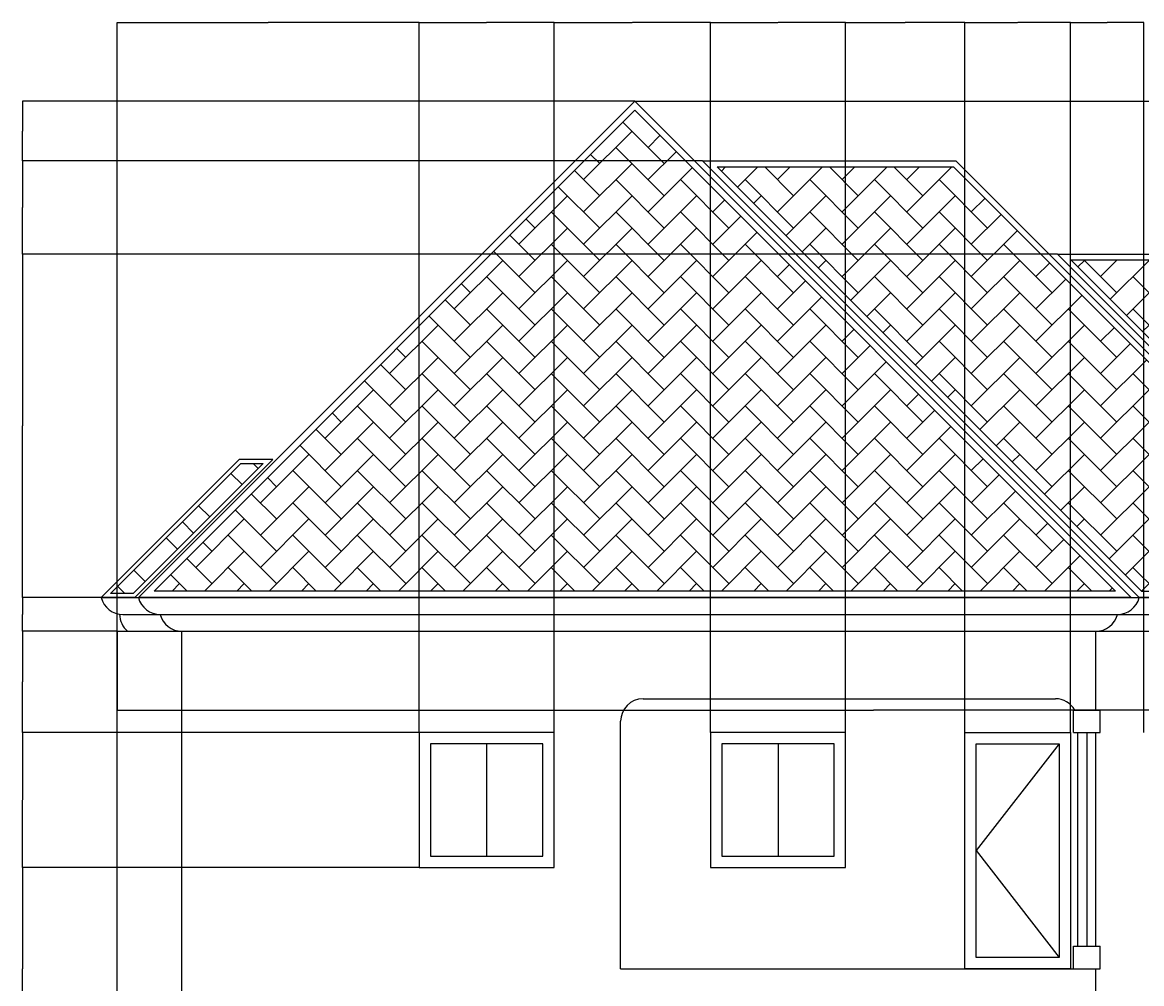
# Model space of a CAD drawing. Units: millimetres. Extents: x 19292 to 100733, y 12374 to 26974.
# Tile 24 of 24: x 85594 to 95547, y 18427 to 26974. Entities that reach past the tile are written whole.
import ezdxf

# ---------------------------------------------------------------- set-up
doc = ezdxf.new("R2010")
doc.units = ezdxf.units.MM
for name, color, linetype, lineweight in [('A-ANNO-DIMS', 2, 'Continuous', 18), ('A-ELEV', 7, 'Continuous', 25), ('A-ELEV-PATT', 8, 'Continuous', 13)]:
    doc.layers.add(name, color=color, linetype=linetype, lineweight=lineweight)
doc.styles.get("Standard").update_dxf_attribs({"font": 'arial.ttf'})
doc.dimstyles.get("Standard").update_dxf_attribs({"dimtxt": 0.18, "dimasz": 0.18, "dimexe": 0.18, "dimexo": 0.0625, "dimgap": 0.09, "dimtad": 0, "dimtih": 1, "dimtoh": 1, "dimdec": 4, "dimzin": 0, "dimdsep": 46, "dimtxsty": 'Standard', "dimcen": 0.09, "dimadec": 0, "dimazin": 0, "dimtfac": 1, "dimtdec": 4, "dimtofl": 0, "dimtmove": 0, "dimatfit": 3, "dimfxl": 1, "dimtolj": 1, "dimtzin": 0, "dimarcsym": 0})

# ---------------------------------------------------------------- blocks, each defined once
blk = doc.blocks.new('WIN-ELEV-1200')
blk.add_line((599.9999832836038, 1100.000156100592), (599.9999832836038, 100.000156100592))
for points in [[(1199.999983283604, 1200.000156100592), (1199.999983283604, 0.0001561005919939), (-1.67163962033e-05, 0.0001561005919939), (-1.67163962033e-05, 1200.000156100592)], [(1099.999983283604, 1100.000156100592), (1099.999983283604, 100.000156100592), (99.9999832836038, 100.000156100592), (99.9999832836038, 1100.000156100592)]]:
    blk.add_lwpolyline(points, close=True)
blk = doc.blocks.new('*D144')
at = {"layer": 'A-ANNO-DIMS', "color": 0, "lineweight": -2, "transparency": 16777216}
for p, q in [((89121.76770300003, 19459.90915600001), (85593.98509100005, 19459.90915600001)), ((85594.16509100008, 19459.72915600001), (85594.16509100008, 18560.0910591378)), ((85594.16509100008, 17660.08915600001), (85594.16509100008, 18559.72725286222)), ((89236.95448300001, 17659.90915600001), (85593.98509100005, 17659.90915600001))]:
    blk.add_line(p, q, dxfattribs=at)
at = {"layer": 'A-ANNO-DIMS', "color": 0, "transparency": 16777216}
for points in [[(85594.13509100005, 19459.72915600001), (85594.19509100006, 19459.72915600001), (85594.16509100008, 19459.90915600001)], [(85594.13509100005, 17660.08915600001), (85594.19509100006, 17660.08915600001), (85594.16509100008, 17659.90915600001)]]:
    blk.add_solid(points, dxfattribs=at)
at = {"layer": 'Defpoints', "color": 0, "transparency": 16777216}
for p in [(85594.16509100008, 19459.90915600001), (89121.83020300003, 19459.90915600001), (89237.01698300002, 17659.90915600001)]:
    blk.add_point(p, dxfattribs=at)
at = {"layer": 'A-ANNO-DIMS', "color": 0, "transparency": 16777216, "insert": (85594.16509100005, 18559.90915599998), "char_height": 0.18, "attachment_point": 5}
blk.add_mtext('\\A1;1800', dxfattribs=at)
blk = doc.blocks.new('*D145')
at = {"layer": 'A-ANNO-DIMS', "color": 0, "lineweight": -2, "transparency": 16777216}
for p, q in [((89121.76770300003, 20659.90915600001), (85593.98509100005, 20659.90915600001)), ((85594.16509100008, 20659.72915600001), (85594.16509100008, 20060.0910591378)), ((85594.16509100008, 19460.08915600001), (85594.16509100008, 20059.72725286222)), ((89121.76770300003, 19459.90915600001), (85593.98509100005, 19459.90915600001))]:
    blk.add_line(p, q, dxfattribs=at)
at = {"layer": 'A-ANNO-DIMS', "color": 0, "transparency": 16777216}
for points in [[(85594.13509100005, 20659.72915600001), (85594.19509100006, 20659.72915600001), (85594.16509100008, 20659.90915600001)], [(85594.13509100005, 19460.08915600001), (85594.19509100006, 19460.08915600001), (85594.16509100008, 19459.90915600001)]]:
    blk.add_solid(points, dxfattribs=at)
at = {"layer": 'Defpoints', "color": 0, "transparency": 16777216}
for p in [(85594.16509100008, 20659.90915600001), (89121.83020300003, 20659.90915600001), (89121.83020300003, 19459.90915600001)]:
    blk.add_point(p, dxfattribs=at)
at = {"layer": 'A-ANNO-DIMS', "color": 0, "transparency": 16777216, "insert": (85594.16509100005, 20059.90915599999), "char_height": 0.18, "attachment_point": 5}
blk.add_mtext('\\A1;1200', dxfattribs=at)
blk = doc.blocks.new('*D146')
at = {"layer": 'A-ANNO-DIMS', "color": 0, "lineweight": -2, "transparency": 16777216}
for p, q in [((86437.75175800003, 21559.90915600001), (85593.98509100005, 21559.90915600001)), ((85594.16509100008, 21559.72915600001), (85594.16509100008, 21110.0910591378)), ((85594.16509100008, 20660.08915600001), (85594.16509100008, 21109.72725286222)), ((89121.76770300003, 20659.90915600001), (85593.98509100005, 20659.90915600001))]:
    blk.add_line(p, q, dxfattribs=at)
at = {"layer": 'A-ANNO-DIMS', "color": 0, "transparency": 16777216}
for points in [[(85594.13509100005, 21559.72915600001), (85594.19509100006, 21559.72915600001), (85594.16509100008, 21559.90915600001)], [(85594.13509100005, 20660.08915600001), (85594.19509100006, 20660.08915600001), (85594.16509100008, 20659.90915600001)]]:
    blk.add_solid(points, dxfattribs=at)
at = {"layer": 'Defpoints', "color": 0, "transparency": 16777216}
for p in [(85594.16509100008, 21559.90915600001), (86437.81425800003, 21559.90915600001), (89121.83020300003, 20659.90915600001)]:
    blk.add_point(p, dxfattribs=at)
at = {"layer": 'A-ANNO-DIMS', "color": 0, "transparency": 16777216, "insert": (85594.16509100005, 21109.90915599999), "char_height": 0.18, "attachment_point": 5}
blk.add_mtext('\\A1;900', dxfattribs=at)
blk = doc.blocks.new('*D147')
at = {"layer": 'A-ANNO-DIMS', "color": 0, "lineweight": -2, "transparency": 16777216}
for p, q in [((86294.10259100003, 21859.90915600001), (85593.98509100005, 21859.90915600001)), ((85594.16509100008, 21859.72915600001), (85594.16509100008, 21710.09112052934)), ((85594.16509100008, 21560.08915600001), (85594.16509100008, 21709.72719147068)), ((86437.75175800003, 21559.90915600001), (85593.98509100005, 21559.90915600001))]:
    blk.add_line(p, q, dxfattribs=at)
at = {"layer": 'A-ANNO-DIMS', "color": 0, "transparency": 16777216}
for points in [[(85594.13509100005, 21859.72915600001), (85594.19509100006, 21859.72915600001), (85594.16509100008, 21859.90915600001)], [(85594.13509100005, 21560.08915600001), (85594.19509100006, 21560.08915600001), (85594.16509100008, 21559.90915600001)]]:
    blk.add_solid(points, dxfattribs=at)
at = {"layer": 'Defpoints', "color": 0, "transparency": 16777216}
for p in [(85594.16509100008, 21859.90915600001), (86294.16509100003, 21859.90915600001), (86437.81425800003, 21559.90915600001)]:
    blk.add_point(p, dxfattribs=at)
at = {"layer": 'A-ANNO-DIMS', "color": 0, "transparency": 16777216, "insert": (85594.16509100005, 21709.90915599998), "char_height": 0.18, "attachment_point": 5}
blk.add_mtext('\\A1;300', dxfattribs=at)
blk = doc.blocks.new('*D148')
at = {"layer": 'A-ANNO-DIMS', "color": 0, "lineweight": -2, "transparency": 16777216}
for p, q in [((94798.25936700004, 24912.22737000001), (85593.98509100005, 24912.22737000001)), ((85594.16509100008, 24912.04737000001), (85594.16509100008, 23386.25022752934)), ((85594.16509100008, 21860.08915600001), (85594.16509100008, 23385.88629847067)), ((86294.10259100003, 21859.90915600001), (85593.98509100005, 21859.90915600001))]:
    blk.add_line(p, q, dxfattribs=at)
at = {"layer": 'A-ANNO-DIMS', "color": 0, "transparency": 16777216}
for points in [[(85594.13509100005, 24912.04737000001), (85594.19509100006, 24912.04737000001), (85594.16509100008, 24912.22737000001)], [(85594.13509100005, 21860.08915600001), (85594.19509100006, 21860.08915600001), (85594.16509100008, 21859.90915600001)]]:
    blk.add_solid(points, dxfattribs=at)
at = {"layer": 'Defpoints', "color": 0, "transparency": 16777216}
for p in [(85594.16509100008, 24912.22737000001), (94798.32186700004, 24912.22737000001), (86294.16509100003, 21859.90915600001)]:
    blk.add_point(p, dxfattribs=at)
at = {"layer": 'A-ANNO-DIMS', "color": 0, "transparency": 16777216, "insert": (85594.16509100005, 23386.06826299999), "char_height": 0.18, "attachment_point": 5}
blk.add_mtext('\\A1;3052.3', dxfattribs=at)
blk = doc.blocks.new('*D149')
at = {"layer": 'A-ANNO-DIMS', "color": 0, "lineweight": -2, "transparency": 16777216}
for p, q in [((91642.59139800003, 25742.60711800001), (85593.98509100005, 25742.60711800001)), ((85594.16509100008, 25742.42711800001), (85594.16509100008, 25327.59920852934)), ((85594.16509100008, 24912.40737000001), (85594.16509100008, 25327.23527947068)), ((94798.25936700004, 24912.22737000001), (85593.98509100005, 24912.22737000001))]:
    blk.add_line(p, q, dxfattribs=at)
at = {"layer": 'A-ANNO-DIMS', "color": 0, "transparency": 16777216}
for points in [[(85594.13509100005, 25742.42711800001), (85594.19509100006, 25742.42711800001), (85594.16509100008, 25742.60711800001)], [(85594.13509100005, 24912.40737000001), (85594.19509100006, 24912.40737000001), (85594.16509100008, 24912.22737000001)]]:
    blk.add_solid(points, dxfattribs=at)
at = {"layer": 'Defpoints', "color": 0, "transparency": 16777216}
for p in [(85594.16509100008, 25742.60711800001), (91642.65389800003, 25742.60711800001), (94798.32186700004, 24912.22737000001)]:
    blk.add_point(p, dxfattribs=at)
at = {"layer": 'A-ANNO-DIMS', "color": 0, "transparency": 16777216, "insert": (85594.16509100005, 25327.41724399998), "char_height": 0.18, "attachment_point": 5}
blk.add_mtext('\\A1;830.4', dxfattribs=at)
blk = doc.blocks.new('*D150')
at = {"layer": 'A-ANNO-DIMS', "color": 0, "lineweight": -2, "transparency": 16777216}
for p, q in [((91039.43747500001, 26274.21100900001), (85593.98509100005, 26274.21100900001)), ((85594.16509100008, 26274.03100900001), (85594.16509100008, 26008.59102802934)), ((85594.16509100008, 25742.78711800001), (85594.16509100008, 26008.22709897068)), ((91642.59139800003, 25742.60711800001), (85593.98509100005, 25742.60711800001))]:
    blk.add_line(p, q, dxfattribs=at)
at = {"layer": 'A-ANNO-DIMS', "color": 0, "transparency": 16777216}
for points in [[(85594.13509100005, 26274.03100900001), (85594.19509100006, 26274.03100900001), (85594.16509100008, 26274.21100900001)], [(85594.13509100005, 25742.78711800001), (85594.19509100006, 25742.78711800001), (85594.16509100008, 25742.60711800001)]]:
    blk.add_solid(points, dxfattribs=at)
at = {"layer": 'Defpoints', "color": 0, "transparency": 16777216}
for p in [(85594.16509100008, 26274.21100900001), (91039.49997500001, 26274.21100900001), (91642.65389800003, 25742.60711800001)]:
    blk.add_point(p, dxfattribs=at)
at = {"layer": 'A-ANNO-DIMS', "color": 0, "transparency": 16777216, "insert": (85594.16509100005, 26008.40906349998), "char_height": 0.18, "attachment_point": 5}
blk.add_mtext('\\A1;531.6', dxfattribs=at)
blk = doc.blocks.new('*D151')
at = {"layer": 'A-ANNO-DIMS', "color": 0, "lineweight": -2, "transparency": 16777216}
for p, q in [((91039.56247500001, 26274.21100900001), (100732.6942110001, 26274.21100900001)), ((100732.5142110001, 26274.03100900001), (100732.5142110001, 20692.2419856378)), ((100732.5142110001, 15110.08915600001), (100732.5142110001, 20691.87817936222)), ((99927.91327500006, 15109.909156), (100732.6942110001, 15109.909156))]:
    blk.add_line(p, q, dxfattribs=at)
at = {"layer": 'A-ANNO-DIMS', "color": 0, "transparency": 16777216}
for points in [[(100732.4842110001, 26274.03100900001), (100732.5442110001, 26274.03100900001), (100732.5142110001, 26274.21100900001)], [(100732.4842110001, 15110.08915600001), (100732.5442110001, 15110.08915600001), (100732.5142110001, 15109.909156)]]:
    blk.add_solid(points, dxfattribs=at)
at = {"layer": 'Defpoints', "color": 0, "transparency": 16777216}
for p in [(91039.49997500001, 26274.21100900001), (100732.5142110001, 26274.21100900001), (99927.85077500006, 15109.909156)]:
    blk.add_point(p, dxfattribs=at)
at = {"layer": 'A-ANNO-DIMS', "color": 0, "transparency": 16777216, "insert": (100732.5142110001, 20692.06008249997), "char_height": 0.18, "attachment_point": 5}
blk.add_mtext('\\A1;11164', dxfattribs=at)
blk = doc.blocks.new('*D161')
at = {"layer": 'A-ANNO-DIMS', "color": 0, "lineweight": -2, "transparency": 16777216}
for p, q in [((86437.814258, 21559.971656), (86437.814258, 26974.391009)), ((86437.99425799999, 26974.211009), (87779.46229189154, 26974.211009)), ((89121.65020300001, 26974.211009), (87780.18216910846, 26974.211009)), ((89121.830203, 20659.971656), (89121.830203, 26974.391009))]:
    blk.add_line(p, q, dxfattribs=at)
at = {"layer": 'A-ANNO-DIMS', "color": 0, "transparency": 16777216}
for points in [[(86437.99425799999, 26974.241009), (86437.99425799999, 26974.181009), (86437.814258, 26974.211009)], [(89121.65020300001, 26974.241009), (89121.65020300001, 26974.181009), (89121.830203, 26974.211009)]]:
    blk.add_solid(points, dxfattribs=at)
at = {"layer": 'Defpoints', "color": 0, "transparency": 16777216}
for p in [(89121.830203, 26974.211009), (86437.814258, 21559.909156), (89121.830203, 20659.909156)]:
    blk.add_point(p, dxfattribs=at)
at = {"layer": 'A-ANNO-DIMS', "color": 0, "transparency": 16777216, "insert": (87779.8222305, 26974.211009), "char_height": 0.18, "attachment_point": 5}
blk.add_mtext('\\A1;2684', dxfattribs=at)
blk = doc.blocks.new('*D162')
at = {"layer": 'A-ANNO-DIMS', "color": 0, "lineweight": -2, "transparency": 16777216}
for p, q in [((89121.830203, 20659.971656), (89121.830203, 26974.391009)), ((89122.01020299998, 26974.211009), (89721.48020982128, 26974.211009)), ((90321.650203, 26974.211009), (89722.18019617873, 26974.211009)), ((90321.830203, 20659.971656), (90321.830203, 26974.391009))]:
    blk.add_line(p, q, dxfattribs=at)
at = {"layer": 'A-ANNO-DIMS', "color": 0, "transparency": 16777216}
for points in [[(89122.01020299998, 26974.241009), (89122.01020299998, 26974.181009), (89121.830203, 26974.211009)], [(90321.650203, 26974.241009), (90321.650203, 26974.181009), (90321.830203, 26974.211009)]]:
    blk.add_solid(points, dxfattribs=at)
at = {"layer": 'Defpoints', "color": 0, "transparency": 16777216}
for p in [(90321.830203, 26974.211009), (89121.830203, 20659.909156), (90321.830203, 20659.909156)]:
    blk.add_point(p, dxfattribs=at)
at = {"layer": 'A-ANNO-DIMS', "color": 0, "transparency": 16777216, "insert": (89721.830203, 26974.211009), "char_height": 0.18, "attachment_point": 5}
blk.add_mtext('\\A1;1200', dxfattribs=at)
blk = doc.blocks.new('*D163')
at = {"layer": 'A-ANNO-DIMS', "color": 0, "lineweight": -2, "transparency": 16777216}
for p, q in [((90321.830203, 20659.971656), (90321.830203, 26974.391009)), ((90322.010203, 26974.211009), (91017.16552300206, 26974.211009)), ((91713.23103400003, 26974.211009), (91018.07571399795, 26974.211009)), ((91713.411034, 20659.971656), (91713.411034, 26974.391009))]:
    blk.add_line(p, q, dxfattribs=at)
at = {"layer": 'A-ANNO-DIMS', "color": 0, "transparency": 16777216}
for points in [[(90322.010203, 26974.241009), (90322.010203, 26974.181009), (90321.830203, 26974.211009)], [(91713.23103400003, 26974.241009), (91713.23103400003, 26974.181009), (91713.411034, 26974.211009)]]:
    blk.add_solid(points, dxfattribs=at)
at = {"layer": 'Defpoints', "color": 0, "transparency": 16777216}
for p in [(91713.411034, 26974.211009), (90321.830203, 20659.909156), (91713.411034, 20659.909156)]:
    blk.add_point(p, dxfattribs=at)
at = {"layer": 'A-ANNO-DIMS', "color": 0, "transparency": 16777216, "insert": (91017.6206185, 26974.211009), "char_height": 0.18, "attachment_point": 5}
blk.add_mtext('\\A1;1391.6', dxfattribs=at)
blk = doc.blocks.new('*D164')
at = {"layer": 'A-ANNO-DIMS', "color": 0, "lineweight": -2, "transparency": 16777216}
for p, q in [((91713.411034, 20659.971656), (91713.411034, 26974.391009)), ((91713.591034, 26974.211009), (92313.06104082127, 26974.211009)), ((92913.23103400001, 26974.211009), (92313.76102717873, 26974.211009)), ((92913.411034, 20659.971656), (92913.411034, 26974.391009))]:
    blk.add_line(p, q, dxfattribs=at)
at = {"layer": 'A-ANNO-DIMS', "color": 0, "transparency": 16777216}
for points in [[(91713.591034, 26974.241009), (91713.591034, 26974.181009), (91713.411034, 26974.211009)], [(92913.23103400001, 26974.241009), (92913.23103400001, 26974.181009), (92913.411034, 26974.211009)]]:
    blk.add_solid(points, dxfattribs=at)
at = {"layer": 'Defpoints', "color": 0, "transparency": 16777216}
for p in [(92913.411034, 26974.211009), (91713.411034, 20659.909156), (92913.411034, 20659.909156)]:
    blk.add_point(p, dxfattribs=at)
at = {"layer": 'A-ANNO-DIMS', "color": 0, "transparency": 16777216, "insert": (92313.411034, 26974.211009), "char_height": 0.18, "attachment_point": 5}
blk.add_mtext('\\A1;1200', dxfattribs=at)
blk = doc.blocks.new('*D165')
at = {"layer": 'A-ANNO-DIMS', "color": 0, "lineweight": -2, "transparency": 16777216}
for p, q in [((92913.411034, 20659.971656), (92913.411034, 26974.391009)), ((92913.59103399998, 26974.211009), (93443.86200193588, 26974.211009)), ((93975.04365200001, 26974.211009), (93444.77268406413, 26974.211009)), ((93975.223652, 20659.971656), (93975.223652, 26974.391009))]:
    blk.add_line(p, q, dxfattribs=at)
at = {"layer": 'A-ANNO-DIMS', "color": 0, "transparency": 16777216}
for points in [[(92913.59103399998, 26974.241009), (92913.59103399998, 26974.181009), (92913.411034, 26974.211009)], [(93975.04365200001, 26974.241009), (93975.04365200001, 26974.181009), (93975.223652, 26974.211009)]]:
    blk.add_solid(points, dxfattribs=at)
at = {"layer": 'Defpoints', "color": 0, "transparency": 16777216}
for p in [(93975.223652, 26974.211009), (92913.411034, 20659.909156), (93975.223652, 20659.909156)]:
    blk.add_point(p, dxfattribs=at)
at = {"layer": 'A-ANNO-DIMS', "color": 0, "transparency": 16777216, "insert": (93444.317343, 26974.211009), "char_height": 0.18, "attachment_point": 5}
blk.add_mtext('\\A1;1061.8', dxfattribs=at)
blk = doc.blocks.new('*D166')
at = {"layer": 'A-ANNO-DIMS', "color": 0, "lineweight": -2, "transparency": 16777216}
for p, q in [((93975.223652, 20659.971656), (93975.223652, 26974.391009)), ((93975.403652, 26974.211009), (94443.90636884993, 26974.211009)), ((94913.16174600001, 26974.211009), (94444.65902915008, 26974.211009)), ((94913.341746, 20659.971656), (94913.341746, 26974.391009))]:
    blk.add_line(p, q, dxfattribs=at)
at = {"layer": 'A-ANNO-DIMS', "color": 0, "transparency": 16777216}
for points in [[(93975.403652, 26974.241009), (93975.403652, 26974.181009), (93975.223652, 26974.211009)], [(94913.16174600001, 26974.241009), (94913.16174600001, 26974.181009), (94913.341746, 26974.211009)]]:
    blk.add_solid(points, dxfattribs=at)
at = {"layer": 'Defpoints', "color": 0, "transparency": 16777216}
for p in [(94913.341746, 26974.211009), (93975.223652, 20659.909156), (94913.341746, 20659.909156)]:
    blk.add_point(p, dxfattribs=at)
at = {"layer": 'A-ANNO-DIMS', "color": 0, "transparency": 16777216, "insert": (94444.282699, 26974.211009), "char_height": 0.18, "attachment_point": 5}
blk.add_mtext('\\A1;938.1', dxfattribs=at)
blk = doc.blocks.new('*D167')
at = {"layer": 'A-ANNO-DIMS', "color": 0, "lineweight": -2, "transparency": 16777216}
for p, q in [((94913.341746, 20659.971656), (94913.341746, 26974.391009)), ((94913.52174600001, 26974.211009), (95240.02142701363, 26974.211009)), ((95567.099048, 26974.211009), (95240.59936698635, 26974.211009)), ((95567.279048, 20659.971656), (95567.279048, 26974.391009))]:
    blk.add_line(p, q, dxfattribs=at)
at = {"layer": 'A-ANNO-DIMS', "color": 0, "transparency": 16777216}
for points in [[(94913.52174600001, 26974.241009), (94913.52174600001, 26974.181009), (94913.341746, 26974.211009)], [(95567.099048, 26974.241009), (95567.099048, 26974.181009), (95567.279048, 26974.211009)]]:
    blk.add_solid(points, dxfattribs=at)
at = {"layer": 'Defpoints', "color": 0, "transparency": 16777216}
for p in [(95567.279048, 26974.211009), (94913.341746, 20659.909156), (95567.279048, 20659.909156)]:
    blk.add_point(p, dxfattribs=at)
at = {"layer": 'A-ANNO-DIMS', "color": 0, "transparency": 16777216, "insert": (95240.310397, 26974.211009), "char_height": 0.18, "attachment_point": 5}
blk.add_mtext('\\A1;654', dxfattribs=at)
blk = doc.blocks.new('*D170')
at = {"layer": 'A-ANNO-DIMS', "color": 0, "lineweight": -2, "transparency": 16777216}
for p, q in [((86437.814258, 21559.846656), (86437.814258, 20859.729156)), ((99888.865044, 21559.846656), (99888.865044, 20859.729156)), ((86437.99425799999, 20859.909156), (93162.93679970397, 20859.909156)), ((99888.685044, 20859.909156), (93163.74250229605, 20859.909156))]:
    blk.add_line(p, q, dxfattribs=at)
at = {"layer": 'A-ANNO-DIMS', "color": 0, "transparency": 16777216}
for points in [[(86437.99425799999, 20859.939156), (86437.99425799999, 20859.879156), (86437.814258, 20859.909156)], [(99888.685044, 20859.939156), (99888.685044, 20859.879156), (99888.865044, 20859.909156)]]:
    blk.add_solid(points, dxfattribs=at)
at = {"layer": 'Defpoints', "color": 0, "transparency": 16777216}
for p in [(86437.814258, 21559.909156), (99888.865044, 21559.909156), (86437.814258, 20859.909156)]:
    blk.add_point(p, dxfattribs=at)
at = {"layer": 'A-ANNO-DIMS', "color": 0, "transparency": 16777216, "insert": (93163.339651, 20859.909156), "char_height": 0.18, "attachment_point": 5}
blk.add_mtext('\\A1;13451', dxfattribs=at)

msp = doc.modelspace()

# ---------------------------------------------------------------- hatches: boundary and pattern name
at = {"layer": 'A-ELEV-PATT'}
h = msp.add_hatch(dxfattribs=at)
h.set_pattern_fill('AR-HBONE', color=256, scale=2)
h.set_pattern_definition([(45, (-15742.66734838602, 1.819e-12), (0, 287.3681958742129), [609.6, -203.2]), (135, (-15598.98334838602, 143.6840000000018), (2.84e-14, 287.3681958742129), [609.6, -203.2])])
h.paths.add_polyline_path([(87735.48117691663, 23052.98438420805), (87536.44885016952, 23052.98438420805), (86378.42981350586, 21894.96534754441), (86578.07896417224, 21895.58217146364)])
h.paths.add_polyline_path([(91039.49997476467, 26192.70967510026), (86764.32960140108, 21917.5393017367), (95314.67034812817, 21917.5393017367)])
h.paths.add_polyline_path([(93872.96419886049, 25688.93910166301), (91772.21995210611, 25688.939101663), (95547.96497158404, 21913.19408218505), (97648.70921833848, 21913.19408218505)])
h.paths.add_polyline_path([(96958.92150424178, 24862.64804519888), (94918.01694600363, 24862.64804519888), (97871.17317701879, 21909.49181418373), (99911.74658381855, 21909.82296562213)])

# ---------------------------------------------------------------- linework, layer by layer
at = {"layer": 'A-ELEV'}
for p, q in [((91642.65389804375, 25742.60711847878), (93895.19421929128, 25742.60711847879)), ((87819.48539444181, 23087.78007040352), (87522.03600503529, 23087.78007040352)), ((86294.16509073348, 21859.90915610059), (100032.5142111294, 21859.90915610059)), ((86487.81425804386, 21709.9091561006), (99838.86504381908, 21709.90915610059)), ((86437.81425804387, 18559.90915610059), (86437.81425804387, 21559.90915610059)), ((86437.81425804387, 21559.90915610059), (99888.8650438191, 21559.90915610059)), ((87012.49645682552, 15559.90915610059), (87012.49645682552, 21559.90915610059)), ((95138.48032185201, 20859.90915610059), (95138.48032185201, 21559.90915610059)), ((91113.34174630335, 20959.90915610059), (94780.028686983, 20959.90915610059)), ((94940.02868698297, 20859.90915610059), (95178.48032185201, 20859.90915610059)), ((94940.02868698297, 20659.90915610059), (94940.02868698297, 20859.90915610059)), ((95178.48032185201, 20659.90915610059), (95178.48032185201, 20859.90915610059)), ((90913.34174630335, 18559.90915610059), (90913.34174630335, 20759.90915610059)), ((94940.02868698297, 20659.90915610059), (95178.48032185201, 20659.90915610059)), ((94980.02868698302, 18759.90915610059), (94980.02868698302, 20659.90915610059)), ((95059.25450441749, 20659.90915610059), (95059.2545044175, 18759.90915610059)), ((95138.48032185201, 18759.90915610059), (95138.48032185201, 20659.90915610059)), ((94813.34174630335, 20559.90915610059), (94075.22365204261, 19609.90915610059)), ((94075.22365204261, 19609.90915610059), (94813.34174630335, 18659.90915610059)), ((94940.02868698302, 18559.90915610059), (94940.02868698302, 18759.90915610059)), ((94940.02868698302, 18759.90915610059), (95178.48032185201, 18759.90915610059)), ((95178.48032185201, 18559.90915610059), (95178.48032185201, 18759.90915610059)), ((86437.81425804387, 15559.90915610059), (86437.81425804387, 18559.90915610059)), ((90913.34174630335, 18559.90915610059), (94940.02868698302, 18559.90915610059)), ((93975.22365204261, 18559.90915610059), (95178.48032185201, 18559.90915610059)), ((93975.22365204261, 18559.90915610059), (95178.48032185201, 18559.90915610059)), ((95138.48032185201, 17859.90915610059), (95138.48032185201, 18559.90915610059))]:
    msp.add_line(p, q, dxfattribs=at)
for points in [[(95453.8018273245, 21859.90915610058), (86625.1981222048, 21859.90915610058), (91039.49997476467, 26274.21100866041), (95453.8018273245, 21859.90915610058)], [(93895.19421929128, 25742.60711847879), (97778.27527240079, 21859.52606536928), (95525.73495115327, 21859.52606536928), (91642.65389804375, 25742.60711847878)], [(96979.45793317242, 24912.22737044603), (100031.422242509, 21860.26306110946), (97850.6400809241, 21859.90915610059), (94798.32186657867, 24912.22737044603), (96979.45793317242, 24912.22737044603)], [(87819.48539444181, 23087.78007040352), (86592.53630977905, 21860.83098574075), (86294.16509073233, 21859.90915610059), (87522.03600503529, 23087.78007040352)]]:
    msp.add_lwpolyline(points, dxfattribs=at)
for points in [[(95314.67034812817, 21917.5393017367), (86764.32960140108, 21917.5393017367), (91039.49997476467, 26192.70967510026)], [(93872.96419886049, 25688.93910166301), (97648.70921833848, 21913.19408218505), (95547.96497158404, 21913.19408218505), (91772.21995210611, 25688.939101663)], [(96958.92150424178, 24862.64804519888), (99911.74658381855, 21909.82296562213), (97871.17317701879, 21909.49181418373), (94918.01694600363, 24862.64804519888)], [(87735.48117691663, 23052.98438420805), (86578.07896417224, 21895.58217146364), (86378.42981350586, 21894.96534754441), (87536.44885016952, 23052.98438420805)], [(93975.22365204261, 20659.90915610059), (94913.34174630335, 20659.90915610059), (94913.34174630335, 18559.90915610059), (93975.22365204261, 18559.90915610059)], [(94075.22365204261, 20559.90915610059), (94813.34174630335, 20559.90915610059), (94813.34174630335, 18659.90915610059), (94075.22365204261, 18659.90915610059)]]:
    msp.add_lwpolyline(points, close=True, dxfattribs=at)
for centre, start, end in [((86487.81425804386, 21909.90915610059), 194.4775121859409, 270), ((86818.84728951516, 21909.9091561006), 194.4775121859407, 270), ((95332.12948916238, 21909.90915610059), 270, 345.5224878140552), ((86658.30467906188, 21712.09817372523), 180, 229.5475857537149), ((87012.49645682552, 21759.90915610059), 194.4775121859161, 270), ((95138.48032185201, 21759.90915610059), 270, 345.5224878140829), ((91113.34174630335, 20759.90915610059), 90, 180), ((94780.028686983, 20759.90915610059), 30.00000000009106, 90)]:
    msp.add_arc(centre, 200, start, end, dxfattribs=at)

# ---------------------------------------------------------------- block references
at = {"layer": 'A-ELEV', "extrusion": (0, 0, -1), "zscale": -1}
for p in [(-90321.83018601831, 19459.90900000001), (-92913.41101736129, 19459.90900000001)]:
    msp.add_blockref('WIN-ELEV-1200', p, dxfattribs=at)

# ---------------------------------------------------------------- dimensions: what is measured, and where the dimension line sits
at = {"layer": 'A-ANNO-DIMS'}
for base, p1, p2, override, picture, middle in [((89121.830203, 26974.211009), (86437.814258, 21559.909156), (89121.830203, 20659.909156), {"dimdec": 0, "dimlfac": 1, "dimrnd": 0, "dimzin": 0, "dimdsep": 46, "dimlunit": 2}, '*D161', (87779.8222305, 26974.211009)), ((90321.830203, 26974.211009), (89121.830203, 20659.909156), (90321.830203, 20659.909156), {"dimdec": 0, "dimlfac": 1, "dimrnd": 0, "dimzin": 0, "dimdsep": 46, "dimlunit": 2}, '*D162', (89721.830203, 26974.211009)), ((91713.411034, 26974.211009), (90321.830203, 20659.909156), (91713.411034, 20659.909156), {"dimdec": 1, "dimlfac": 1, "dimrnd": 0, "dimzin": 0, "dimdsep": 46, "dimlunit": 2}, '*D163', (91017.6206185, 26974.211009)), ((92913.411034, 26974.211009), (91713.411034, 20659.909156), (92913.411034, 20659.909156), {"dimdec": 0, "dimlfac": 1, "dimrnd": 0, "dimzin": 0, "dimdsep": 46, "dimlunit": 2}, '*D164', (92313.411034, 26974.211009)), ((93975.223652, 26974.211009), (92913.411034, 20659.909156), (93975.223652, 20659.909156), {"dimdec": 1, "dimlfac": 1, "dimrnd": 0, "dimzin": 0, "dimdsep": 46, "dimlunit": 2}, '*D165', (93444.317343, 26974.211009)), ((94913.341746, 26974.211009), (93975.223652, 20659.909156), (94913.341746, 20659.909156), {"dimdec": 1, "dimlfac": 1, "dimrnd": 0, "dimzin": 0, "dimdsep": 46, "dimlunit": 2}, '*D166', (94444.282699, 26974.211009)), ((95567.279048, 26974.211009), (94913.341746, 20659.909156), (95567.279048, 20659.909156), {"dimdec": 0, "dimlfac": 1, "dimrnd": 0, "dimzin": 0, "dimdsep": 46, "dimlunit": 2}, '*D167', (95240.310397, 26974.211009))]:
    dim = msp.add_linear_dim(base=base, p1=p1, p2=p2, dimstyle='Standard', override=override, dxfattribs=at)
    dim.commit()
    dim.dimension.update_dxf_attribs({"geometry": picture, "text_midpoint": middle})
for base, p1, p2, angle, override, picture, middle in [((85594.16509100008, 26274.21100900001), (91642.653898, 25742.607118), (91039.499975, 26274.211009), 90, {"dimdec": 1, "dimlfac": 1, "dimrnd": 0, "dimzin": 0, "dimdsep": 46, "dimlunit": 2}, '*D150', (85594.16509100005, 26008.40906349998)), ((100732.5142110001, 26274.21100900001), (99927.850775, 15109.909156), (91039.499975, 26274.211009), 90, {"dimdec": 0, "dimlfac": 1, "dimrnd": 0, "dimzin": 0, "dimdsep": 46, "dimlunit": 2}, '*D151', (100732.5142110001, 20692.06008249997)), ((85594.16509100008, 25742.60711800001), (94798.321867, 24912.22737), (91642.653898, 25742.607118), 90, {"dimdec": 1, "dimlfac": 1, "dimrnd": 0, "dimzin": 0, "dimdsep": 46, "dimlunit": 2}, '*D149', (85594.16509100005, 25327.41724399998)), ((85594.16509100008, 24912.22737000001), (86294.165091, 21859.909156), (94798.321867, 24912.22737), 90, {"dimdec": 1, "dimlfac": 1, "dimrnd": 0, "dimzin": 0, "dimdsep": 46, "dimlunit": 2}, '*D148', (85594.16509100005, 23386.06826299999)), ((85594.16509100008, 21859.90915600001), (86437.814258, 21559.909156), (86294.165091, 21859.909156), 90, {"dimdec": 0, "dimlfac": 1, "dimrnd": 0, "dimzin": 0, "dimdsep": 46, "dimlunit": 2}, '*D147', (85594.16509100005, 21709.90915599998)), ((85594.16509100008, 21559.90915600001), (89121.830203, 20659.909156), (86437.814258, 21559.909156), 90, {"dimdec": 0, "dimlfac": 1, "dimrnd": 0, "dimzin": 0, "dimdsep": 46, "dimlunit": 2}, '*D146', (85594.16509100005, 21109.90915599999)), ((86437.814258, 20859.909156), (99888.865044, 21559.909156), (86437.814258, 21559.909156), 180, {"dimdec": 0, "dimlfac": 1, "dimrnd": 0, "dimzin": 0, "dimdsep": 46, "dimlunit": 2}, '*D170', (93163.339651, 20859.909156)), ((85594.16509100008, 20659.90915600001), (89121.830203, 19459.909156), (89121.830203, 20659.909156), 90, {"dimdec": 0, "dimlfac": 1, "dimrnd": 0, "dimzin": 0, "dimdsep": 46, "dimlunit": 2}, '*D145', (85594.16509100005, 20059.90915599999)), ((85594.16509100008, 19459.90915600001), (89237.016983, 17659.909156), (89121.830203, 19459.909156), 90, {"dimdec": 0, "dimlfac": 1, "dimrnd": 0, "dimzin": 0, "dimdsep": 46, "dimlunit": 2}, '*D144', (85594.16509100005, 18559.90915599998))]:
    dim = msp.add_linear_dim(base=base, p1=p1, p2=p2, angle=angle, dimstyle='Standard', override=override, dxfattribs=at)
    dim.commit()
    dim.dimension.update_dxf_attribs({"geometry": picture, "text_midpoint": middle})

doc.saveas('drawing.dxf')
